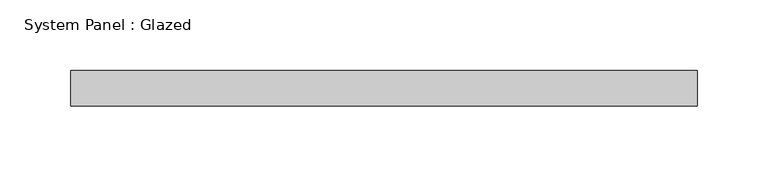
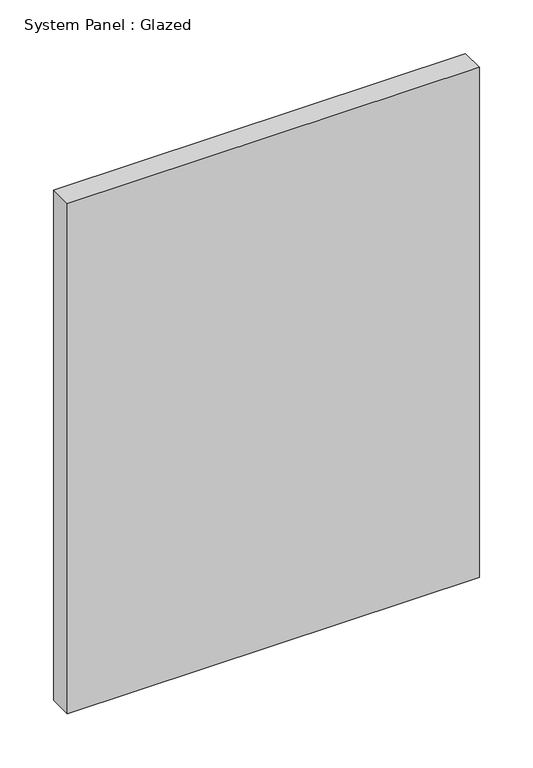
"""IFC4 building model written with IfcOpenShell, lengths in millimetres: plate geometry, System Panel : Glazed."""

from ifc_helpers import new_model, si_unit, origin, origin_with_axes, place, context, project, spatial, polyline, outline, extrude, source, transform, mapped, element, save


def system_panel_glazed_d072c6ac(model_context):
    return source(origin(), model_context, "Body", "SweptSolid", [
        extrude(outline(polyline([(222.25, 19.05), (-222.25, 19.05), (-222.25, 44.45), (222.25, 44.45), (222.25, 19.05)])), origin_with_axes(), (0.0, 0.0, 1.0), 582.0833333),
    ])


if __name__ == "__main__":
    model = new_model("IFC4")
    model_context = context("Model", 3, world=origin())
    ifc_project = project(units=[si_unit("LENGTHUNIT", "METRE", prefix="MILLI")], contexts=[model_context])
    site = spatial("IfcSite", under=ifc_project)
    building = spatial("IfcBuilding", under=site)
    placement = place(None, origin())
    system_panel_glazed_shape = system_panel_glazed_d072c6ac(model_context)
    element("IfcPlate", 1, ObjectType="System Panel : Glazed", at=placement, inside=building, context=model_context, shape_type="MappedRepresentation", body=[
        mapped(system_panel_glazed_shape, transform((0.0, 0.0, 0.0), x_axis=(1.0, 0.0, 0.0), y_axis=(0.0, 1.0, 0.0), z_axis=(0.0, 0.0, 1.0))),
    ])
    save(model, "model.ifc")

# Revit data of these elements
# Type "System Panel : Glazed"
#   Construction Type Id = "GSP4R"
#   Analytic Construction = "1/8 in Pilkington single glazing"
#   Visual Light Transmittance = 0.9
#   Solar Heat Gain Coefficient = 0.86
#   Heat Transfer Coefficient (U) = 1.18115 BTU/(h·ft²·°F)
#   Define Thermal Properties by = 1
# Element 1 (IfcPlate, "System Panel : Glazed")
#   Materials on its faces: "Glass"
# Materials
#   "Glass": class "Glass", colour RGB 0 128 192, transparency 0.75, Description = "Soda Lime Glass", Cost = 0
